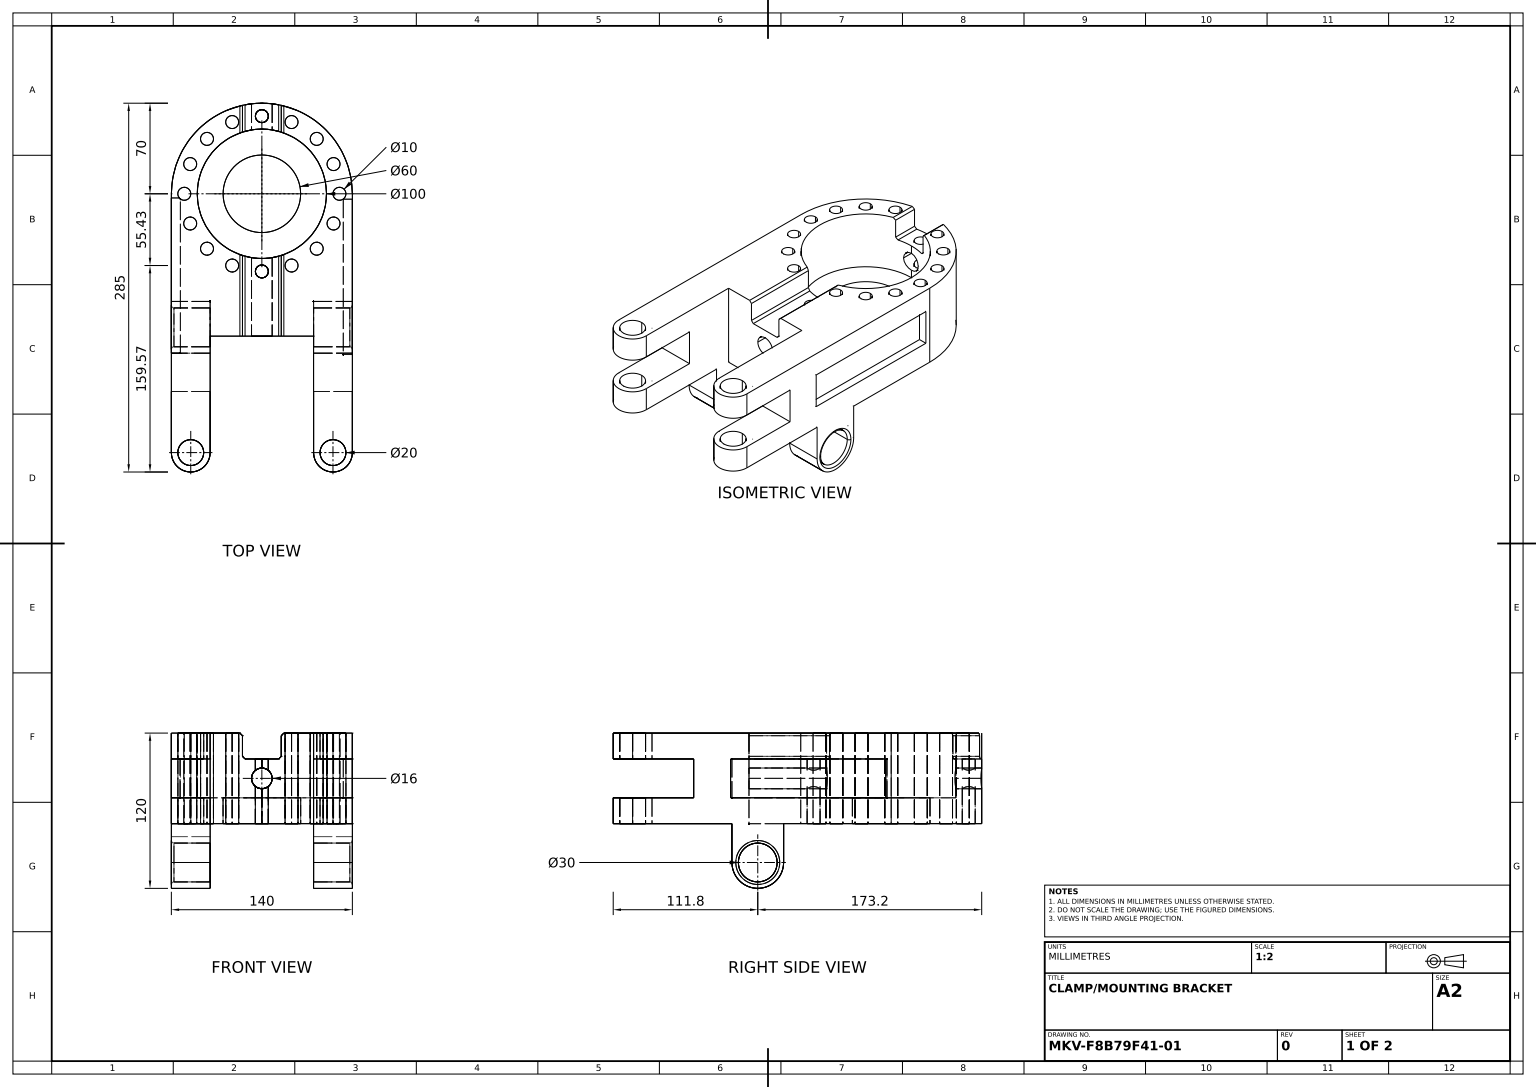
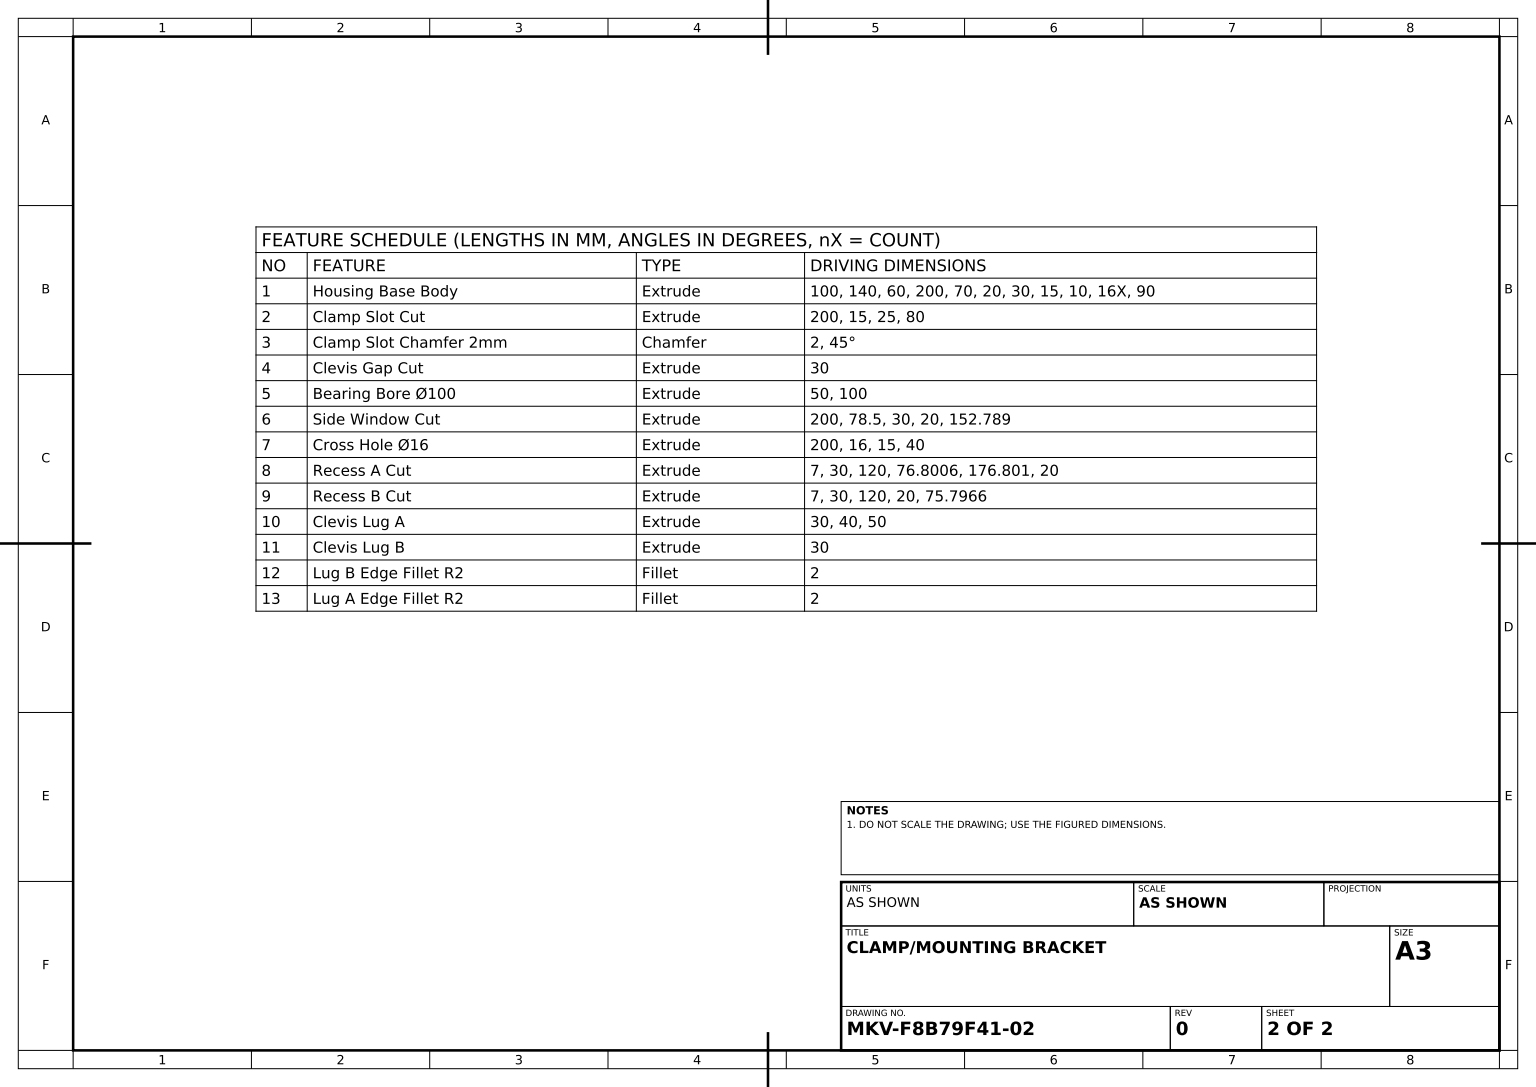
from build123d import *

# Parameters (mm, degrees)
HOUSING_BASE_PROFILE_SKETCH_R   = 30
HOUSING_BASE_PROFILE_SKETCH_R_2 = 10
HOUSING_BASE_PROFILE_SKETCH_R_3 = 5
HOUSING_BASE_BODY_DEPTH         = 100
CLAMP_SLOT_SKETCH_W             = 30
CLAMP_SLOT_SKETCH_H             = 20
CLAMP_SLOT_CUT_DEPTH            = 200
CLAMP_SLOT_CHAMFER_2MM_SIZE     = 2
CLEVIS_GAP_CUT_DEPTH            = 30
BEARING_BORE_SKETCH_R           = 50
BEARING_BORE_100_DEPTH          = 50
SIDE_WINDOW_SKETCH_W            = 47.211428362
SIDE_WINDOW_SKETCH_H            = 30
SIDE_WINDOW_SKETCH_W_2          = 31.288571638
SIDE_WINDOW_CUT_DEPTH           = 200
CROSS_HOLE_SKETCH_R             = 8
CROSS_HOLE_16_DEPTH             = 200
RECESS_A_CUT_DEPTH              = 7
RECESS_B_SKETCH_W               = 120
RECESS_B_SKETCH_H               = 30
RECESS_B_CUT_DEPTH              = 7
CLEVIS_LUG_A_SKETCH_R           = 15
CLEVIS_LUG_A_DEPTH              = 30
CLEVIS_START                    = -30
CLEVIS_LUG_B_SKETCH_R           = 15
CLEVIS_LUG_B_DEPTH              = 30
LUG_B_EDGE_FILLET_R2_R          = 2
LUG_A_EDGE_FILLET_R2_R          = 2


with BuildPart() as part:
    # Housing Base Profile Sketch → Housing Base Body (new body)
    with BuildSketch(Plane(origin=(0, 0, 0), x_dir=(1, 0, 0), z_dir=(0, 1, 0))):
        with BuildLine():
            Line((-70, 200), (-70, 0))
            ThreePointArc((-70, 0), (-55, -15), (-40, 0))
            Line((-40, 0), (-40, 90))
            Line((-40, 90), (40, 90))
            Line((40, 90), (40, 0))
            ThreePointArc((40, 0), (55, -15), (70, 0))
            Line((70, 0), (70, 200))
            ThreePointArc((70, 200), (0, 270), (-70, 200))
        make_face()
        with Locations(Location((0, 200, 0), (0, 0, 270))):
            Circle(HOUSING_BASE_PROFILE_SKETCH_R, mode=Mode.SUBTRACT)
        with Locations(Location((-55, 0, 0), (0, 0, 270))):
            Circle(HOUSING_BASE_PROFILE_SKETCH_R_2, mode=Mode.SUBTRACT)
        with Locations(Location((55, 0, 0), (0, 0, 270))):
            Circle(HOUSING_BASE_PROFILE_SKETCH_R_2, mode=Mode.SUBTRACT)
        with Locations(Location((0, 260, 0), (0, 0, 270))):
            Circle(HOUSING_BASE_PROFILE_SKETCH_R_3, mode=Mode.SUBTRACT)
        with Locations(Location((22.961005942, 255.432771951, 0), (0, 0, 270))):
            Circle(HOUSING_BASE_PROFILE_SKETCH_R_3, mode=Mode.SUBTRACT)
        with Locations(Location((42.426406871, 242.426406871, 0), (0, 0, 270))):
            Circle(HOUSING_BASE_PROFILE_SKETCH_R_3, mode=Mode.SUBTRACT)
        with Locations(Location((55.432771951, 222.961005942, 0), (0, 0, 270))):
            Circle(HOUSING_BASE_PROFILE_SKETCH_R_3, mode=Mode.SUBTRACT)
        with Locations(Location((60, 200, 0), (0, 0, 270))):
            Circle(HOUSING_BASE_PROFILE_SKETCH_R_3, mode=Mode.SUBTRACT)
        with Locations(Location((55.432771951, 177.038994058, 0), (0, 0, 270))):
            Circle(HOUSING_BASE_PROFILE_SKETCH_R_3, mode=Mode.SUBTRACT)
        with Locations(Location((42.426406871, 157.573593129, 0), (0, 0, 270))):
            Circle(HOUSING_BASE_PROFILE_SKETCH_R_3, mode=Mode.SUBTRACT)
        with Locations(Location((22.961005942, 144.567228049, 0), (0, 0, 270))):
            Circle(HOUSING_BASE_PROFILE_SKETCH_R_3, mode=Mode.SUBTRACT)
        with Locations(Location((0, 140, 0), (0, 0, 270))):
            Circle(HOUSING_BASE_PROFILE_SKETCH_R_3, mode=Mode.SUBTRACT)
        with Locations(Location((-22.961005942, 144.567228049, 0), (0, 0, 270))):
            Circle(HOUSING_BASE_PROFILE_SKETCH_R_3, mode=Mode.SUBTRACT)
        with Locations(Location((-42.426406871, 157.573593129, 0), (0, 0, 270))):
            Circle(HOUSING_BASE_PROFILE_SKETCH_R_3, mode=Mode.SUBTRACT)
        with Locations(Location((-55.432771951, 177.038994058, 0), (0, 0, 270))):
            Circle(HOUSING_BASE_PROFILE_SKETCH_R_3, mode=Mode.SUBTRACT)
        with Locations(Location((-60, 200, 0), (0, 0, 270))):
            Circle(HOUSING_BASE_PROFILE_SKETCH_R_3, mode=Mode.SUBTRACT)
        with Locations(Location((-55.432771951, 222.961005942, 0), (0, 0, 270))):
            Circle(HOUSING_BASE_PROFILE_SKETCH_R_3, mode=Mode.SUBTRACT)
        with Locations(Location((-42.426406871, 242.426406871, 0), (0, 0, 270))):
            Circle(HOUSING_BASE_PROFILE_SKETCH_R_3, mode=Mode.SUBTRACT)
        with Locations(Location((-22.961005942, 255.432771951, 0), (0, 0, 270))):
            Circle(HOUSING_BASE_PROFILE_SKETCH_R_3, mode=Mode.SUBTRACT)
    extrude(amount=HOUSING_BASE_BODY_DEPTH)

    # Clamp Slot Sketch → Clamp Slot Cut (cut)
    with BuildSketch(Plane.XY.offset(-90)):
        with Locations((0, 90)):
            Rectangle(CLAMP_SLOT_SKETCH_W, CLAMP_SLOT_SKETCH_H)
    extrude(amount=-CLAMP_SLOT_CUT_DEPTH, mode=Mode.SUBTRACT)

    # Clamp Slot Chamfer 2mm
    clamp_slot_chamfer_2mm_edges = [part.edges().sort_by_distance(p)[0] for p in [
        (15, 100, -247.177366885),
        (-15, 80, -247.177366885),
        (15, 80, -247.177366885),
        (15, 80, -132.009618943),
        (-15, 100, -247.177366885),
        (15, 100, -132.009618943),
        (-15, 80, -132.009618943),
        (-15, 100, -132.009618943),
    ]]
    chamfer(clamp_slot_chamfer_2mm_edges, length=CLAMP_SLOT_CHAMFER_2MM_SIZE)

    # Clevis Gap Sketch → Clevis Gap Cut (cut)
    with BuildSketch(Plane.XZ):
        with BuildLine():
            Line((-70, 0), (-70, -200))
            ThreePointArc((-70, -200), (0, -270), (70, -200))
            Line((70, -200), (70, 0))
            ThreePointArc((70, 0), (55, 15), (40, 0))
            Line((40, 0), (40, -90))
            Line((40, -90), (-40, -90))
            Line((-40, -90), (-40, 0))
            ThreePointArc((-40, 0), (-55, 15), (-70, 0))
        make_face()
    extrude(amount=-CLEVIS_GAP_CUT_DEPTH, mode=Mode.SUBTRACT)

    # Bearing Bore Sketch → Bearing Bore Ø100 (cut)
    with BuildSketch(Plane(origin=(0, 100, 0), x_dir=(1, 0, 0), z_dir=(0, 1, 0))):
        with Locations(Location((0, 200, 0), (0, 0, 270))):
            Circle(BEARING_BORE_SKETCH_R)
    extrude(amount=-BEARING_BORE_100_DEPTH, mode=Mode.SUBTRACT)

    # Side Window Sketch → Side Window Cut (cut)
    with BuildSketch(Plane.ZY.offset(70)):
        with Locations((-23.605714181, 65)):
            Rectangle(SIDE_WINDOW_SKETCH_W, SIDE_WINDOW_SKETCH_H)
        with Locations((15.644285819, 65)):
            Rectangle(SIDE_WINDOW_SKETCH_W_2, SIDE_WINDOW_SKETCH_H)
    extrude(amount=-SIDE_WINDOW_CUT_DEPTH, mode=Mode.SUBTRACT)

    # Cross Hole Sketch → Cross Hole Ø16 (cut)
    with BuildSketch(Plane.XY.offset(-90)):
        with Locations((0, 65)):
            Circle(CROSS_HOLE_SKETCH_R)
    extrude(amount=-CROSS_HOLE_16_DEPTH, mode=Mode.SUBTRACT)

    # Recess A Sketch → Recess A Cut (cut)
    with BuildSketch(Plane.ZY.offset(70)):
        Polygon((-76.800577584, 50), (-76.800577584, 80), (-176.800577584, 80), (-196.800577584, 80), (-196.800577584, 50), (-176.800577584, 50), align=None)
    extrude(amount=-RECESS_A_CUT_DEPTH, mode=Mode.SUBTRACT)

    # Recess B Sketch → Recess B Cut (cut)
    with BuildSketch(Plane(origin=(70, 0, 0), x_dir=(0, 0, -1), z_dir=(1, 0, 0))):
        with Locations((135.796628626, 65)):
            Rectangle(RECESS_B_SKETCH_W, RECESS_B_SKETCH_H)
    extrude(amount=-RECESS_B_CUT_DEPTH, mode=Mode.SUBTRACT)

    # Clevis Lug A Sketch → Clevis Lug A (add)
    with BuildSketch(Plane.ZY.offset(70)):
        with BuildLine():
            Line((-76.800577584, 50), (-76.800577584, 0))
            ThreePointArc((-76.800577584, 0), (-96.800577584, -20), (-116.800577584, 0))
            Line((-116.800577584, 0), (-116.800577584, 50))
            Line((-116.800577584, 50), (-76.800577584, 50))
        make_face()
        with Locations((-96.800577584, 0)):
            Circle(CLEVIS_LUG_A_SKETCH_R, mode=Mode.SUBTRACT)
    extrude(amount=-CLEVIS_LUG_A_DEPTH)

    # Clevis Lug B Sketch → Clevis Lug B (add)
    with BuildSketch(Plane(origin=(70, 0, 0), x_dir=(0, 0, -1), z_dir=(1, 0, 0)).offset(CLEVIS_START)):
        with BuildLine():
            Line((76.800577584, 30), (116.800577584, 30))
            Line((116.800577584, 30), (116.800577584, 0))
            ThreePointArc((116.800577584, 0), (96.800577584, -20), (76.800577584, 0))
            Line((76.800577584, 0), (76.800577584, 30))
        make_face()
        with Locations(Location((96.800577584, 0, 0), (0, 0, 180))):
            Circle(CLEVIS_LUG_B_SKETCH_R, mode=Mode.SUBTRACT)
    extrude(amount=CLEVIS_LUG_B_DEPTH)

    # Lug B Edge Fillet R2
    lug_b_edge_fillet_r2_edges = [part.edges().sort_by_distance(p)[0] for p in [
        (70, 0, -111.800577584),
    ]]
    fillet(lug_b_edge_fillet_r2_edges, radius=LUG_B_EDGE_FILLET_R2_R)

    # Lug A Edge Fillet R2
    lug_a_edge_fillet_r2_edges = [part.edges().sort_by_distance(p)[0] for p in [
        (-70, 0, -111.800577584),
    ]]
    fillet(lug_a_edge_fillet_r2_edges, radius=LUG_A_EDGE_FILLET_R2_R)


solid = part.part
